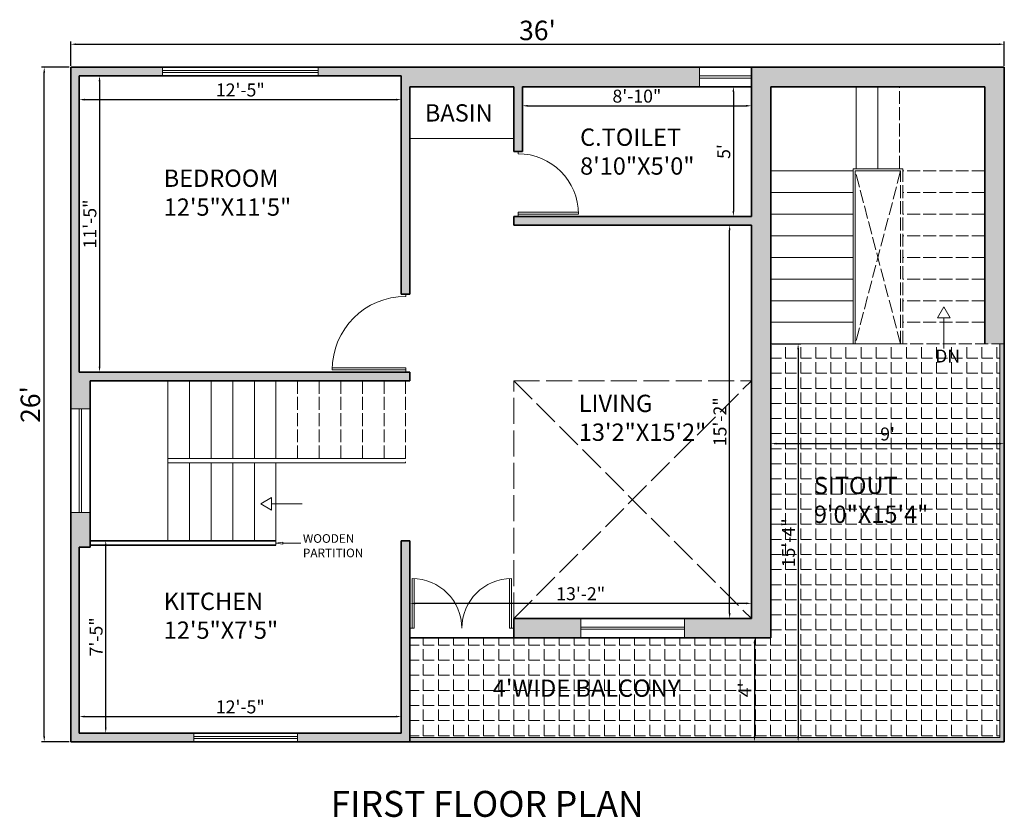
# Model space of a CAD drawing. Units: inches. Extents: x 1947 to 4744, y 610 to 1869.
# Tile 6 of 8: x 4265 to 4720, y 1074 to 1443. Entities that reach past the tile are written whole.
import ezdxf

# ---------------------------------------------------------------- set-up
doc = ezdxf.new("R2010")
doc.units = ezdxf.units.IN
doc.linetypes.add('ACAD_ISO02W100', pattern=[15, 12, -3])
for name, color, linetype, lineweight in [('A-ANNO-DIMS', 2, 'Continuous', 18), ('A-ANNO-SYMB', 2, 'Continuous', 18), ('A-ANNO-TEXT', 7, 'Continuous', 18), ('A-ANNO-TITL', 7, 'Continuous', 35), ('A-AREA-IDEN', 7, 'Continuous', 18), ('A-DOOR', 3, 'Continuous', 18), ('A-FLOR-FIXT', 9, 'Continuous', 18), ('A-FLOR-OPEN-PROJ', 8, 'ACAD_ISO02W100', 13), ('A-FLOR-STRS', 7, 'Continuous', 18), ('A-FLOR-STRS-OVHD', 7, 'ACAD_ISO02W100', 13), ('A-GLAZ', 4, 'Continuous', 18), ('A-WALL', 7, 'Continuous', 35), ('A-WALL-PRHT', 7, 'Continuous', 18)]:
    doc.layers.add(name, color=color, linetype=linetype, lineweight=lineweight)
doc.layers.add('A-FLOR-PATT', color=251, linetype='Continuous', lineweight=13, true_color=0x636466)
doc.layers.add('A-WALL-PATT', color=18, linetype='Continuous', lineweight=13, true_color=0x000000)
doc.styles.get("Standard").update_dxf_attribs({"font": 'arial.ttf'})
doc.dimstyles.new('ISO-25', dxfattribs={"dimtxt": 9, "dimasz": 2.5, "dimexe": 1.25, "dimexo": 0.625, "dimtad": 1, "dimdec": 1, "dimlunit": 3, "dimtxsty": 'Standard', "dimcen": 2.5, "dimadec": 0, "dimazin": 0, "dimtfac": 1, "dimtdec": 1, "dimtmove": 0, "dimatfit": 3, "dimfxl": 1, "dimarcsym": 0})

# ---------------------------------------------------------------- blocks, each defined once
blk = doc.blocks.new('1')
for p, q in [((4267.36, 1627.82), (4267.36, 1650.82)), ((4268.36, 1627.82), (4268.36, 1650.82)), ((4312.36, 1627.82), (4312.36, 1650.82)), ((4313.36, 1627.82), (4313.36, 1650.82)), ((4266.36, 1627.82), (4268.36, 1627.82)), ((4314.36, 1627.82), (4312.36, 1627.82))]:
    blk.add_line(p, q)
at = {"ltscale": 0.5}
for centre, start, end in [((4267.36, 1627.82), 0, 90), ((4313.36, 1627.82), 90, 180)]:
    blk.add_arc(centre, 23, start, end, dxfattribs=at)
blk = doc.blocks.new('2')
for p, q in [((4319.45, 1679.18), (4319.45, 1713.18)), ((4320.45, 1679.18), (4320.45, 1713.18)), ((4318.45, 1679.18), (4320.45, 1679.18)), ((4353.45, 1679.18), (4354.45, 1679.18))]:
    blk.add_line(p, q)
at = {"ltscale": 0.5}
blk.add_arc((4319.45, 1679.18), 34, 0, 90, dxfattribs=at)
blk = doc.blocks.new('4')
for p, q in [((3808.6, 1693.11), (3808.6, 1721.11)), ((3809.6, 1693.11), (3809.6, 1721.11)), ((3807.6, 1693.11), (3809.6, 1693.11)), ((3836.6, 1693.11), (3837.6, 1693.11))]:
    blk.add_line(p, q)
at = {"ltscale": 0.5}
blk.add_arc((3808.6, 1693.11), 28, 0, 90, dxfattribs=at)
blk = doc.blocks.new('*D13')
at = {"layer": 'A-ANNO-DIMS', "color": 0, "lineweight": -2, "transparency": 16777216}
for p, q in [((4287.57, 1420.79), (4274.7, 1420.79)), ((4275.95, 1111.29), (4275.95, 1418.29)), ((4287.57, 1108.79), (4274.7, 1108.79))]:
    blk.add_line(p, q, dxfattribs=at)
at = {"layer": 'A-ANNO-DIMS', "color": 0, "transparency": 16777216}
for points in [[(4275.54, 1418.29), (4276.37, 1418.29), (4275.95, 1420.79)], [(4275.54, 1111.29), (4276.37, 1111.29), (4275.95, 1108.79)]]:
    blk.add_solid(points, dxfattribs=at)
at = {"layer": 'Defpoints', "color": 0, "transparency": 16777216}
for p in [(4275.95, 1420.79), (4288.19, 1420.79), (4288.19, 1108.79)]:
    blk.add_point(p, dxfattribs=at)
at = {"layer": 'A-ANNO-DIMS', "color": 0, "transparency": 16777216, "insert": (4270.73, 1264.79), "char_height": 9, "attachment_point": 5, "rotation": 90}
blk.add_mtext("26'", dxfattribs=at)
blk = doc.blocks.new('*D14')
at = {"layer": 'A-ANNO-DIMS', "color": 0, "lineweight": -2, "transparency": 16777216}
for p, q in [((4288.19, 1421.41), (4288.19, 1432.67)), ((4290.69, 1431.42), (4717.69, 1431.42)), ((4720.19, 1421.41), (4720.19, 1432.67))]:
    blk.add_line(p, q, dxfattribs=at)
at = {"layer": 'A-ANNO-DIMS', "color": 0, "transparency": 16777216}
for points in [[(4290.69, 1431.83), (4290.69, 1431), (4288.19, 1431.42)], [(4717.69, 1431.83), (4717.69, 1431), (4720.19, 1431.42)]]:
    blk.add_solid(points, dxfattribs=at)
at = {"layer": 'Defpoints', "color": 0, "transparency": 16777216}
for p in [(4720.19, 1431.42), (4288.19, 1420.79), (4720.19, 1420.79)]:
    blk.add_point(p, dxfattribs=at)
at = {"layer": 'A-ANNO-DIMS', "color": 0, "transparency": 16777216, "insert": (4504.19, 1436.64), "char_height": 9, "attachment_point": 5}
blk.add_mtext("36'", dxfattribs=at)
blk = doc.blocks.new('*D35')
at = {"layer": 'A-ANNO-DIMS', "color": 0, "lineweight": -2, "transparency": 16777216}
for p, q in [((4292.82, 1416.79), (4302.8, 1416.79)), ((4301.55, 1414.29), (4301.55, 1282.29)), ((4292.82, 1279.79), (4302.8, 1279.79))]:
    blk.add_line(p, q, dxfattribs=at)
at = {"layer": 'A-ANNO-DIMS', "color": 0, "transparency": 16777216}
for points in [[(4301.13, 1414.29), (4301.97, 1414.29), (4301.55, 1416.79)], [(4301.13, 1282.29), (4301.97, 1282.29), (4301.55, 1279.79)]]:
    blk.add_solid(points, dxfattribs=at)
at = {"layer": 'Defpoints', "color": 0, "transparency": 16777216}
for p in [(4292.19, 1416.79), (4292.19, 1279.79), (4301.55, 1279.79)]:
    blk.add_point(p, dxfattribs=at)
at = {"layer": 'A-ANNO-DIMS', "color": 0, "transparency": 16777216, "insert": (4297.86, 1348.29), "char_height": 6, "attachment_point": 5, "rotation": 90}
blk.add_mtext('11\'-5"', dxfattribs=at)
blk = doc.blocks.new('*D36')
at = {"layer": 'A-ANNO-DIMS', "color": 0, "lineweight": -2, "transparency": 16777216}
for p, q in [((4292.19, 1416.16), (4292.19, 1404.55)), ((4441.19, 1416.16), (4441.19, 1404.55)), ((4294.69, 1405.8), (4438.69, 1405.8))]:
    blk.add_line(p, q, dxfattribs=at)
at = {"layer": 'A-ANNO-DIMS', "color": 0, "transparency": 16777216}
for points in [[(4294.69, 1406.22), (4294.69, 1405.38), (4292.19, 1405.8)], [(4438.69, 1406.22), (4438.69, 1405.38), (4441.19, 1405.8)]]:
    blk.add_solid(points, dxfattribs=at)
at = {"layer": 'Defpoints', "color": 0, "transparency": 16777216}
for p in [(4292.19, 1416.79), (4441.19, 1416.79), (4441.19, 1405.8)]:
    blk.add_point(p, dxfattribs=at)
at = {"layer": 'A-ANNO-DIMS', "color": 0, "transparency": 16777216, "insert": (4366.69, 1409.49), "char_height": 6, "attachment_point": 5}
blk.add_mtext('12\'-5"', dxfattribs=at)
blk = doc.blocks.new('*D37')
at = {"layer": 'A-ANNO-DIMS', "color": 0, "lineweight": -2, "transparency": 16777216}
for p, q in [((4497.19, 1411.16), (4497.19, 1401.7)), ((4603.19, 1411.16), (4603.19, 1401.7)), ((4499.69, 1402.95), (4600.69, 1402.95))]:
    blk.add_line(p, q, dxfattribs=at)
at = {"layer": 'A-ANNO-DIMS', "color": 0, "transparency": 16777216}
for points in [[(4499.69, 1403.36), (4499.69, 1402.53), (4497.19, 1402.95)], [(4600.69, 1403.36), (4600.69, 1402.53), (4603.19, 1402.95)]]:
    blk.add_solid(points, dxfattribs=at)
at = {"layer": 'Defpoints', "color": 0, "transparency": 16777216}
for p in [(4497.19, 1411.79), (4603.19, 1411.79), (4603.19, 1402.95)]:
    blk.add_point(p, dxfattribs=at)
at = {"layer": 'A-ANNO-DIMS', "color": 0, "transparency": 16777216, "insert": (4550.19, 1406.64), "char_height": 6, "attachment_point": 5}
blk.add_mtext('8\'-10"', dxfattribs=at)
blk = doc.blocks.new('*D38')
at = {"layer": 'A-ANNO-DIMS', "color": 0, "lineweight": -2, "transparency": 16777216}
for p, q in [((4602.57, 1411.79), (4593.59, 1411.79)), ((4594.84, 1409.29), (4594.84, 1354.29)), ((4602.57, 1351.79), (4593.59, 1351.79))]:
    blk.add_line(p, q, dxfattribs=at)
at = {"layer": 'A-ANNO-DIMS', "color": 0, "transparency": 16777216}
for points in [[(4594.43, 1409.29), (4595.26, 1409.29), (4594.84, 1411.79)], [(4594.43, 1354.29), (4595.26, 1354.29), (4594.84, 1351.79)]]:
    blk.add_solid(points, dxfattribs=at)
at = {"layer": 'Defpoints', "color": 0, "transparency": 16777216}
for p in [(4603.19, 1411.79), (4594.84, 1351.79), (4603.19, 1351.79)]:
    blk.add_point(p, dxfattribs=at)
at = {"layer": 'A-ANNO-DIMS', "color": 0, "transparency": 16777216, "insert": (4591.17, 1381.79), "char_height": 6, "attachment_point": 5, "rotation": 90}
blk.add_mtext("5'", dxfattribs=at)
blk = doc.blocks.new('*D39')
at = {"layer": 'A-ANNO-DIMS', "color": 0, "lineweight": -2, "transparency": 16777216}
for p, q in [((4297.82, 1201.79), (4305.66, 1201.79)), ((4304.41, 1115.29), (4304.41, 1199.29)), ((4297.82, 1112.79), (4305.66, 1112.79))]:
    blk.add_line(p, q, dxfattribs=at)
at = {"layer": 'A-ANNO-DIMS', "color": 0, "transparency": 16777216}
for points in [[(4303.99, 1199.29), (4304.83, 1199.29), (4304.41, 1201.79)], [(4303.99, 1115.29), (4304.83, 1115.29), (4304.41, 1112.79)]]:
    blk.add_solid(points, dxfattribs=at)
at = {"layer": 'Defpoints', "color": 0, "transparency": 16777216}
for p in [(4297.19, 1201.79), (4304.41, 1201.79), (4297.19, 1112.79)]:
    blk.add_point(p, dxfattribs=at)
at = {"layer": 'A-ANNO-DIMS', "color": 0, "transparency": 16777216, "insert": (4300.73, 1157.29), "char_height": 6, "attachment_point": 5, "rotation": 90}
blk.add_mtext('7\'-5"', dxfattribs=at)
blk = doc.blocks.new('*D40')
at = {"layer": 'A-ANNO-DIMS', "color": 0, "lineweight": -2, "transparency": 16777216}
for p, q in [((4292.19, 1113.41), (4292.19, 1121.68)), ((4441.19, 1113.41), (4441.19, 1121.68)), ((4294.69, 1120.43), (4438.69, 1120.43))]:
    blk.add_line(p, q, dxfattribs=at)
at = {"layer": 'A-ANNO-DIMS', "color": 0, "transparency": 16777216}
for points in [[(4294.69, 1120.85), (4294.69, 1120.01), (4292.19, 1120.43)], [(4438.69, 1120.85), (4438.69, 1120.01), (4441.19, 1120.43)]]:
    blk.add_solid(points, dxfattribs=at)
at = {"layer": 'Defpoints', "color": 0, "transparency": 16777216}
for p in [(4441.19, 1120.43), (4292.19, 1112.79), (4441.19, 1112.79)]:
    blk.add_point(p, dxfattribs=at)
at = {"layer": 'A-ANNO-DIMS', "color": 0, "transparency": 16777216, "insert": (4366.69, 1124.12), "char_height": 6, "attachment_point": 5}
blk.add_mtext('12\'-5"', dxfattribs=at)
blk = doc.blocks.new('*D41')
at = {"layer": 'A-ANNO-DIMS', "color": 0, "lineweight": -2, "transparency": 16777216}
for p, q in [((4445.19, 1166.41), (4445.19, 1174.04)), ((4600.69, 1172.79), (4447.69, 1172.79)), ((4603.19, 1166.41), (4603.19, 1174.04))]:
    blk.add_line(p, q, dxfattribs=at)
at = {"layer": 'A-ANNO-DIMS', "color": 0, "transparency": 16777216}
for points in [[(4447.69, 1173.21), (4447.69, 1172.37), (4445.19, 1172.79)], [(4600.69, 1173.21), (4600.69, 1172.37), (4603.19, 1172.79)]]:
    blk.add_solid(points, dxfattribs=at)
at = {"layer": 'Defpoints', "color": 0, "transparency": 16777216}
for p in [(4445.19, 1172.79), (4445.19, 1165.79), (4603.19, 1165.79)]:
    blk.add_point(p, dxfattribs=at)
at = {"layer": 'A-ANNO-DIMS', "color": 0, "transparency": 16777216, "insert": (4524.19, 1176.48), "char_height": 6, "attachment_point": 5}
blk.add_mtext('13\'-2"', dxfattribs=at)
blk = doc.blocks.new('*D42')
at = {"layer": 'A-ANNO-DIMS', "color": 0, "lineweight": -2, "transparency": 16777216}
for p, q in [((4602.57, 1347.79), (4591.85, 1347.79)), ((4593.1, 1168.29), (4593.1, 1345.29)), ((4602.57, 1165.79), (4591.85, 1165.79))]:
    blk.add_line(p, q, dxfattribs=at)
at = {"layer": 'A-ANNO-DIMS', "color": 0, "transparency": 16777216}
for points in [[(4592.68, 1345.29), (4593.51, 1345.29), (4593.1, 1347.79)], [(4592.68, 1168.29), (4593.51, 1168.29), (4593.1, 1165.79)]]:
    blk.add_solid(points, dxfattribs=at)
at = {"layer": 'Defpoints', "color": 0, "transparency": 16777216}
for p in [(4593.1, 1347.79), (4603.19, 1347.79), (4603.19, 1165.79)]:
    blk.add_point(p, dxfattribs=at)
at = {"layer": 'A-ANNO-DIMS', "color": 0, "transparency": 16777216, "insert": (4589.41, 1256.79), "char_height": 6, "attachment_point": 5, "rotation": 90}
blk.add_mtext('15\'-2"', dxfattribs=at)
blk = doc.blocks.new('*D43')
at = {"layer": 'A-ANNO-DIMS', "color": 0, "lineweight": -2, "transparency": 16777216}
for p, q in [((4612.19, 1250.99), (4612.19, 1245.43)), ((4720.19, 1250.99), (4720.19, 1245.43)), ((4614.69, 1246.68), (4717.69, 1246.68))]:
    blk.add_line(p, q, dxfattribs=at)
at = {"layer": 'A-ANNO-DIMS', "color": 0, "transparency": 16777216}
for points in [[(4614.69, 1247.09), (4614.69, 1246.26), (4612.19, 1246.68)], [(4717.69, 1247.09), (4717.69, 1246.26), (4720.19, 1246.68)]]:
    blk.add_solid(points, dxfattribs=at)
at = {"layer": 'Defpoints', "color": 0, "transparency": 16777216}
for p in [(4612.19, 1251.61), (4720.19, 1251.61), (4720.19, 1246.68)]:
    blk.add_point(p, dxfattribs=at)
at = {"layer": 'A-ANNO-DIMS', "color": 0, "transparency": 16777216, "insert": (4666.19, 1250.36), "char_height": 6, "attachment_point": 5}
blk.add_mtext("9'", dxfattribs=at)
blk = doc.blocks.new('*D44')
at = {"layer": 'A-ANNO-DIMS', "color": 0, "lineweight": -2, "transparency": 16777216}
for p, q in [((4612.82, 1292.79), (4626.05, 1292.79)), ((4624.8, 1290.29), (4624.8, 1111.29)), ((4612.82, 1108.79), (4626.05, 1108.79))]:
    blk.add_line(p, q, dxfattribs=at)
at = {"layer": 'A-ANNO-DIMS', "color": 0, "transparency": 16777216}
for points in [[(4624.38, 1290.29), (4625.22, 1290.29), (4624.8, 1292.79)], [(4624.38, 1111.29), (4625.22, 1111.29), (4624.8, 1108.79)]]:
    blk.add_solid(points, dxfattribs=at)
at = {"layer": 'Defpoints', "color": 0, "transparency": 16777216}
for p in [(4612.19, 1292.79), (4612.19, 1108.79), (4624.8, 1108.79)]:
    blk.add_point(p, dxfattribs=at)
at = {"layer": 'A-ANNO-DIMS', "color": 0, "transparency": 16777216, "insert": (4621.11, 1200.79), "char_height": 6, "attachment_point": 5, "rotation": 90}
blk.add_mtext('15\'-4"', dxfattribs=at)
blk = doc.blocks.new('*D45')
at = {"layer": 'A-ANNO-DIMS', "color": 0, "lineweight": -2, "transparency": 16777216}
for p, q in [((4604.57, 1154.29), (4604.57, 1111.29)), ((4605.2, 1156.79), (4605.82, 1156.79)), ((4605.2, 1108.79), (4605.82, 1108.79))]:
    blk.add_line(p, q, dxfattribs=at)
at = {"layer": 'A-ANNO-DIMS', "color": 0, "transparency": 16777216}
for points in [[(4604.16, 1154.29), (4604.99, 1154.29), (4604.57, 1156.79)], [(4604.16, 1111.29), (4604.99, 1111.29), (4604.57, 1108.79)]]:
    blk.add_solid(points, dxfattribs=at)
at = {"layer": 'Defpoints', "color": 0, "transparency": 16777216}
for p in [(4604.57, 1156.79), (4604.57, 1108.79), (4604.57, 1108.79)]:
    blk.add_point(p, dxfattribs=at)
at = {"layer": 'A-ANNO-DIMS', "color": 0, "transparency": 16777216, "insert": (4600.95, 1132.79), "char_height": 6, "attachment_point": 5, "rotation": 90}
blk.add_mtext("4'", dxfattribs=at)
blk = doc.blocks.new('WIN-72-4')
for p, q in [((0, 0), (0, 4)), ((72, 2.5), (0, 2.5)), ((72, 1.5), (0, 1.5)), ((72, 0), (72, 4))]:
    blk.add_line(p, q)
blk = doc.blocks.new('WIN-48-4')
for p, q in [((0, 0), (0, 4)), ((48, 2.5), (0, 2.5)), ((48, 1.5), (0, 1.5)), ((48, 0), (48, 4))]:
    blk.add_line(p, q)
blk = doc.blocks.new('WIN-48-9')
for p, q in [((0, 0), (0, 9)), ((48, 5), (0, 5)), ((48, 0), (48, 9)), ((48, 4), (0, 4))]:
    blk.add_line(p, q)
blk = doc.blocks.new('STAIR-DIRECTION')
blk.add_line((2.91, 14.18), (2.91, 0))
blk.add_lwpolyline([(2.91, 19.23), (0, 14.18), (5.83, 14.18)], close=True)
blk = doc.blocks.new('PARTITION-LEADER')
blk.add_line((3.21, 0.5), (11.48, 0.5))
blk.add_lwpolyline([(0, 0.5), (3.21, 0), (3.21, 0.99)], close=True)

msp = doc.modelspace()

# ---------------------------------------------------------------- hatches: boundary and pattern name
at = {"layer": 'A-FLOR-PATT'}
h = msp.add_hatch(dxfattribs=at)
h.set_pattern_fill('ANGLE', color=256)
h.set_pattern_definition([(0, (574.662, -6.012), (0, 6.985), [5.08, -1.905]), (90, (574.662, -6.012), (-6.985, 4e-16), [5.08, -1.905])])
h.paths.add_polyline_path([(4612.19, 1156.79), (4445.19, 1156.79), (4445.19, 1110.79), (4718.19, 1110.79), (4718.19, 1292.79), (4672.19, 1292.79), (4612.19, 1292.79)])
h.paths.add_polyline_path([(4686.56, 1280.8), (4702.36, 1280.8), (4702.36, 1293.61), (4686.56, 1293.61)], flags=9)
h.paths.add_polyline_path([(4481.32, 1125.02), (4584.23, 1125.02), (4584.23, 1142.1), (4481.32, 1142.1)], flags=24)
h.paths.add_polyline_path([(4629.35, 1205.44), (4685.58, 1205.44), (4685.58, 1235.86), (4629.35, 1235.86)], flags=24)
at = {"layer": 'A-WALL-PATT'}
h = msp.add_hatch(color=256, dxfattribs=at)
h.dxf.hatch_style = 1
h.paths.add_polyline_path([(4445.19, 1279.79), (4292.19, 1279.79), (4292.19, 1416.79), (4330.69, 1416.79), (4330.69, 1420.79), (4288.19, 1420.79), (4288.19, 1262.79), (4297.19, 1262.79), (4297.19, 1275.79), (4445.19, 1275.79)])
h.paths.add_polyline_path([(4297.19, 1214.79), (4288.19, 1214.79), (4288.19, 1108.79), (4345.19, 1108.79), (4345.19, 1112.79), (4292.19, 1112.79), (4292.19, 1198.79), (4297.19, 1198.79)])
h.paths.add_polyline_path([(4445.19, 1201.79), (4441.19, 1201.79), (4441.19, 1112.79), (4393.19, 1112.79), (4393.19, 1108.79), (4445.19, 1108.79)])
h.paths.add_polyline_path([(4524.19, 1165.79), (4493.19, 1165.79), (4493.19, 1156.79), (4524.19, 1156.79)])
h.paths.add_polyline_path([(4612.19, 1411.79), (4711.19, 1411.79), (4711.19, 1292.79), (4720.19, 1292.79), (4720.19, 1420.79), (4603.19, 1420.79), (4603.19, 1351.79), (4493.19, 1351.79), (4493.19, 1347.79), (4603.19, 1347.79), (4603.19, 1165.79), (4572.19, 1165.79), (4572.19, 1156.79), (4612.19, 1156.79)])
h.paths.add_polyline_path([(4579.19, 1420.79), (4402.69, 1420.79), (4402.69, 1416.79), (4441.19, 1416.79), (4441.19, 1315.79), (4445.19, 1315.79), (4445.19, 1411.79), (4493.19, 1411.79), (4493.19, 1381.79), (4497.19, 1381.79), (4497.19, 1411.79), (4579.19, 1411.79)])
h.paths.add_polyline_path([(4720.19, 1292.79), (4718.19, 1292.79), (4718.19, 1110.79), (4720.19, 1110.79)])
h.paths.add_polyline_path([(4718.19, 1110.79), (4445.19, 1110.79), (4445.19, 1108.79), (4718.19, 1108.79)])
h.paths.add_polyline_path([(4720.19, 1110.79), (4718.19, 1110.79), (4718.19, 1108.79), (4720.19, 1108.79)])

# ---------------------------------------------------------------- linework, layer by layer
at = {"layer": 'A-FLOR-FIXT'}
msp.add_line((4493.19, 1387.79), (4445.19, 1387.79), dxfattribs=at)
at = {"layer": 'A-FLOR-OPEN-PROJ'}
for p, q in [((4493.19, 1275.79), (4603.19, 1165.79)), ((4493.19, 1165.79), (4603.19, 1275.79))]:
    msp.add_line(p, q, dxfattribs=at)
msp.add_lwpolyline([(4603.19, 1165.79), (4493.19, 1165.79), (4493.19, 1275.79), (4603.19, 1275.79)], close=True, dxfattribs=at)
at = {"layer": 'A-FLOR-STRS'}
for p, q in [((4651.69, 1373.79), (4651.69, 1411.79)), ((4661.69, 1373.79), (4661.69, 1411.79)), ((4650.19, 1372.79), (4612.19, 1372.79)), ((4673.19, 1373.79), (4650.19, 1373.79)), ((4650.19, 1292.79), (4650.19, 1373.79)), ((4672.19, 1372.79), (4651.19, 1372.79)), ((4651.19, 1292.79), (4651.19, 1372.79)), ((4650.19, 1362.79), (4612.19, 1362.79)), ((4650.19, 1352.79), (4612.19, 1352.79)), ((4650.19, 1342.79), (4612.19, 1342.79)), ((4650.19, 1332.79), (4612.19, 1332.79)), ((4650.19, 1322.79), (4612.19, 1322.79)), ((4650.19, 1312.79), (4612.19, 1312.79)), ((4650.19, 1302.79), (4612.19, 1302.79)), ((4672.19, 1292.79), (4612.19, 1292.79)), ((4333.19, 1275.79), (4333.19, 1201.79)), ((4343.19, 1275.79), (4343.19, 1239.79)), ((4353.19, 1275.79), (4353.19, 1239.79)), ((4363.19, 1275.79), (4363.19, 1239.79)), ((4373.19, 1275.79), (4373.19, 1239.79)), ((4383.19, 1275.79), (4383.19, 1239.79)), ((4443.19, 1239.79), (4333.19, 1239.79)), ((4333.19, 1237.79), (4443.19, 1237.79)), ((4343.19, 1237.79), (4343.19, 1201.79)), ((4353.19, 1237.79), (4353.19, 1201.79)), ((4363.19, 1237.79), (4363.19, 1201.79)), ((4373.19, 1237.79), (4373.19, 1201.79)), ((4383.19, 1237.79), (4383.19, 1199.79))]:
    msp.add_line(p, q, dxfattribs=at)
at = {"layer": 'A-FLOR-STRS-OVHD', "ltscale": 0.5}
for p, q in [((4671.69, 1373.79), (4671.69, 1411.79)), ((4672.19, 1372.79), (4651.19, 1292.79)), ((4672.19, 1292.79), (4651.19, 1372.79)), ((4672.19, 1292.79), (4672.19, 1372.79)), ((4673.19, 1292.79), (4673.19, 1373.79)), ((4711.19, 1372.79), (4673.19, 1372.79)), ((4711.19, 1362.79), (4673.19, 1362.79)), ((4711.19, 1352.79), (4673.19, 1352.79)), ((4711.19, 1342.79), (4673.19, 1342.79)), ((4711.19, 1332.79), (4673.19, 1332.79)), ((4711.19, 1322.79), (4673.19, 1322.79)), ((4711.19, 1312.79), (4673.19, 1312.79)), ((4711.19, 1302.79), (4673.19, 1302.79)), ((4720.19, 1292.79), (4672.19, 1292.79)), ((4393.19, 1275.79), (4393.19, 1239.79)), ((4403.19, 1275.79), (4403.19, 1239.79)), ((4413.19, 1275.79), (4413.19, 1239.79)), ((4423.19, 1275.79), (4423.19, 1239.79)), ((4433.19, 1275.79), (4433.19, 1239.79)), ((4443.19, 1275.79), (4443.19, 1237.79))]:
    msp.add_line(p, q, dxfattribs=at)
at = {"layer": 'A-GLAZ'}
for p, q in [((4579.19, 1411.79), (4579.19, 1420.79)), ((4603.19, 1416.79), (4579.19, 1416.79)), ((4603.19, 1415.79), (4579.19, 1415.79))]:
    msp.add_line(p, q, dxfattribs=at)
at = {"layer": 'A-WALL'}
for p, q in [((4720.19, 1420.79), (4288.19, 1420.79)), ((4288.19, 1420.79), (4288.19, 1108.79)), ((4603.19, 1351.79), (4603.19, 1420.79)), ((4720.19, 1108.79), (4720.19, 1420.79)), ((4441.19, 1416.79), (4292.19, 1416.79)), ((4292.19, 1416.79), (4292.19, 1279.79)), ((4441.19, 1416.79), (4441.19, 1315.79)), ((4493.19, 1411.79), (4445.19, 1411.79)), ((4445.19, 1411.79), (4445.19, 1315.79)), ((4493.19, 1381.79), (4493.19, 1411.79)), ((4603.19, 1411.79), (4497.19, 1411.79)), ((4497.19, 1381.79), (4497.19, 1411.79)), ((4711.19, 1411.79), (4612.19, 1411.79)), ((4612.19, 1156.79), (4612.19, 1411.79)), ((4711.19, 1292.79), (4711.19, 1411.79)), ((4497.19, 1381.79), (4493.19, 1381.79)), ((4603.19, 1351.79), (4493.19, 1351.79)), ((4493.19, 1347.79), (4493.19, 1351.79)), ((4493.19, 1347.79), (4603.19, 1347.79)), ((4603.19, 1165.79), (4603.19, 1347.79)), ((4445.19, 1315.79), (4441.19, 1315.79)), ((4445.19, 1279.79), (4292.19, 1279.79)), ((4445.19, 1275.79), (4297.19, 1275.79)), ((4297.19, 1275.79), (4297.19, 1198.79)), ((4445.19, 1279.79), (4445.19, 1275.79)), ((4292.19, 1198.79), (4292.19, 1112.79)), ((4292.19, 1198.79), (4297.19, 1198.79)), ((4297.19, 1201.79), (4383.19, 1201.79)), ((4297.19, 1199.79), (4383.19, 1199.79)), ((4441.19, 1201.79), (4445.19, 1201.79)), ((4441.19, 1201.79), (4441.19, 1112.79)), ((4445.19, 1201.79), (4445.19, 1108.79)), ((4493.19, 1165.79), (4493.19, 1156.79)), ((4493.19, 1165.79), (4603.19, 1165.79)), ((4445.19, 1156.79), (4612.19, 1156.79)), ((4292.19, 1112.79), (4441.19, 1112.79)), ((4288.19, 1108.79), (4720.19, 1108.79))]:
    msp.add_line(p, q, dxfattribs=at)
at = {"layer": 'A-WALL-PRHT'}
for p, q in [((4718.19, 1110.79), (4718.19, 1292.79)), ((4445.19, 1110.79), (4718.19, 1110.79))]:
    msp.add_line(p, q, dxfattribs=at)

# ---------------------------------------------------------------- block references
at = {"layer": 'A-ANNO-SYMB'}
msp.add_blockref('STAIR-DIRECTION', (4689.28, 1290.71), dxfattribs=at)
at = {"layer": 'A-ANNO-SYMB', "rotation": 90.00000000000095}
msp.add_blockref('STAIR-DIRECTION', (4395.36, 1215.88), dxfattribs=at)
at = {"layer": 'A-ANNO-TEXT'}
msp.add_blockref('PARTITION-LEADER', (4383.19, 1200.17), dxfattribs=at)
at = {"layer": 'A-DOOR', "xscale": -1, "rotation": 270}
msp.add_blockref('4', (2802.08, -2455.81), dxfattribs=at)
at = {"layer": 'A-DOOR', "rotation": 90.00000000000003}
msp.add_blockref('2', (6122.38, -3038.66), dxfattribs=at)
at = {"layer": 'A-DOOR'}
msp.add_blockref('1', (178.83, -466.53), dxfattribs=at)
at = {"layer": 'A-GLAZ'}
for name, p in [('WIN-72-4', (4330.69, 1416.79)), ('WIN-48-9', (4524.19, 1156.79)), ('WIN-48-4', (4345.19, 1108.79))]:
    msp.add_blockref(name, p, dxfattribs=at)
at = {"layer": 'A-GLAZ', "rotation": 270.0000000000002}
msp.add_blockref('WIN-48-9', (4288.19, 1262.79), dxfattribs=at)

# ---------------------------------------------------------------- texts
at = {"layer": 'A-ANNO-TEXT', "attachment_point": 1}
for s, insert, char_height in [('{\\fTimes New Roman|b0|i0|c0|p18;BASIN}', (4452.08, 1403.67), 8), ('{\\fTimes New Roman|b0|i0|c0|p18;DN}', (4688.21, 1290.21), 6), ('{\\fTimes New Roman|b0|i0|c0|p18;WOODEN\\PPARTITION}', (4395.65, 1204.8), 4)]:
    msp.add_mtext_dynamic_manual_height_columns(s, width=158.3328, gutter_width=12.5, heights=[0], dxfattribs=dict(at, insert=insert, char_height=char_height))
at = {"layer": 'A-ANNO-TITL', "insert": (4408.49, 1086.05), "char_height": 12, "attachment_point": 1}
msp.add_mtext_dynamic_manual_height_columns('{\\fTimes New Roman|b0|i0|c0|p18;FIRST FLOOR PLAN}', width=253.4596, gutter_width=12.5, heights=[0], dxfattribs=at)
at = {"layer": 'A-AREA-IDEN', "char_height": 8, "attachment_point": 1}
for s, width, heights, insert in [('{\\fTimes New Roman|b0|i0|c0|p18;C.TOILET\\P8\'10"X5\'0"}', 64.3566, [21.47], (4523.89, 1392.43)), ('{\\fTimes New Roman|b0|i0|c0|p18;BEDROOM\\P12\'5"X11\'5"}', 64.3566, [0], (4331.24, 1373.44)), ('{\\fTimes New Roman|b0|i0|c0|p18;LIVING\\P13\'2"X15\'2"}', 64.3566, [21.47], (4523.29, 1269.3)), ('{\\fTimes New Roman|b0|i0|c0|p18;SITOUT\\P9\'0"X15\'4"}', 64.3566, [0], (4632.08, 1231.33)), ('{\\fTimes New Roman|b0|i0|c0|p18;KITCHEN\\P12\'5"X7\'5"}', 64.3566, [0], (4331.24, 1177.74)), ("{\\fTimes New Roman|b0|i0|c0|p18;4'WIDE BALCONY}", 158.3328, [0], (4483.5, 1137.58))]:
    msp.add_mtext_dynamic_manual_height_columns(s, width=width, gutter_width=12.5, heights=heights, dxfattribs=dict(at, insert=insert))

# ---------------------------------------------------------------- dimensions: what is measured, and where the dimension line sits
at = {"layer": 'A-ANNO-DIMS'}
for base, p1, p2, override, picture, middle in [((4720.19, 1431.42), (4288.19, 1420.79), (4720.19, 1420.79), {"dimclrd": 0, "dimclre": 0, "dimclrt": 0}, '*D14', (4504.19, 1436.64)), ((4441.19, 1405.8), (4292.19, 1416.79), (4441.19, 1416.79), {"dimtxt": 6, "dimclrd": 0, "dimclre": 0, "dimclrt": 0}, '*D36', (4366.69, 1409.49)), ((4603.19, 1402.95), (4497.19, 1411.79), (4603.19, 1411.79), {"dimtxt": 6, "dimclrd": 0, "dimclre": 0, "dimclrt": 0}, '*D37', (4550.19, 1406.64)), ((4720.19, 1246.68), (4612.19, 1251.61), (4720.19, 1251.61), {"dimtxt": 6, "dimclrd": 0, "dimclre": 0, "dimclrt": 0}, '*D43', (4666.19, 1250.36)), ((4445.19, 1172.79), (4603.19, 1165.79), (4445.19, 1165.79), {"dimtxt": 6, "dimclrd": 0, "dimclre": 0, "dimclrt": 0}, '*D41', (4524.19, 1176.48)), ((4441.19, 1120.43), (4292.19, 1112.79), (4441.19, 1112.79), {"dimtxt": 6, "dimclrd": 0, "dimclre": 0, "dimclrt": 0}, '*D40', (4366.69, 1124.12))]:
    dim = msp.add_linear_dim(base=base, p1=p1, p2=p2, dimstyle='ISO-25', override=override, dxfattribs=at)
    dim.commit()
    dim.dimension.update_dxf_attribs({"geometry": picture, "text_midpoint": middle})
for base, p1, p2, override, picture, middle in [((4275.95, 1420.79), (4288.19, 1108.79), (4288.19, 1420.79), {"dimclrd": 0, "dimclre": 0, "dimclrt": 0}, '*D13', (4270.73, 1264.79)), ((4301.55, 1279.79), (4292.19, 1416.79), (4292.19, 1279.79), {"dimtxt": 6, "dimclrd": 0, "dimclre": 0, "dimclrt": 0}, '*D35', (4297.86, 1348.29)), ((4594.84, 1351.79), (4603.19, 1411.79), (4603.19, 1351.79), {"dimtxt": 6, "dimclrd": 0, "dimclre": 0, "dimclrt": 0}, '*D38', (4591.17, 1381.79)), ((4593.1, 1347.79), (4603.19, 1165.79), (4603.19, 1347.79), {"dimtxt": 6, "dimclrd": 0, "dimclre": 0, "dimclrt": 0}, '*D42', (4589.41, 1256.79)), ((4624.8, 1108.79), (4612.19, 1292.79), (4612.19, 1108.79), {"dimtxt": 6, "dimclrd": 0, "dimclre": 0, "dimclrt": 0}, '*D44', (4621.11, 1200.79)), ((4304.41, 1201.79), (4297.19, 1112.79), (4297.19, 1201.79), {"dimtxt": 6, "dimclrd": 0, "dimclre": 0, "dimclrt": 0}, '*D39', (4300.73, 1157.29)), ((4604.57, 1108.79), (4604.57, 1156.79), (4604.57, 1108.79), {"dimtxt": 6, "dimclrd": 0, "dimclre": 0, "dimclrt": 0}, '*D45', (4600.95, 1132.79))]:
    dim = msp.add_linear_dim(base=base, p1=p1, p2=p2, angle=90, dimstyle='ISO-25', override=override, dxfattribs=at)
    dim.commit()
    dim.dimension.update_dxf_attribs({"geometry": picture, "text_midpoint": middle})

doc.saveas('drawing.dxf')
